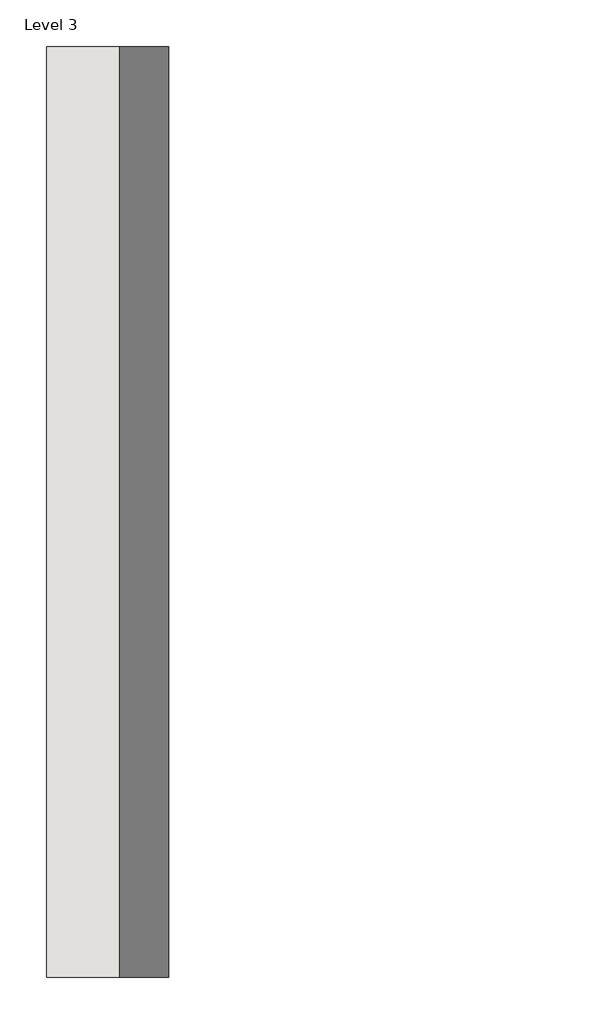
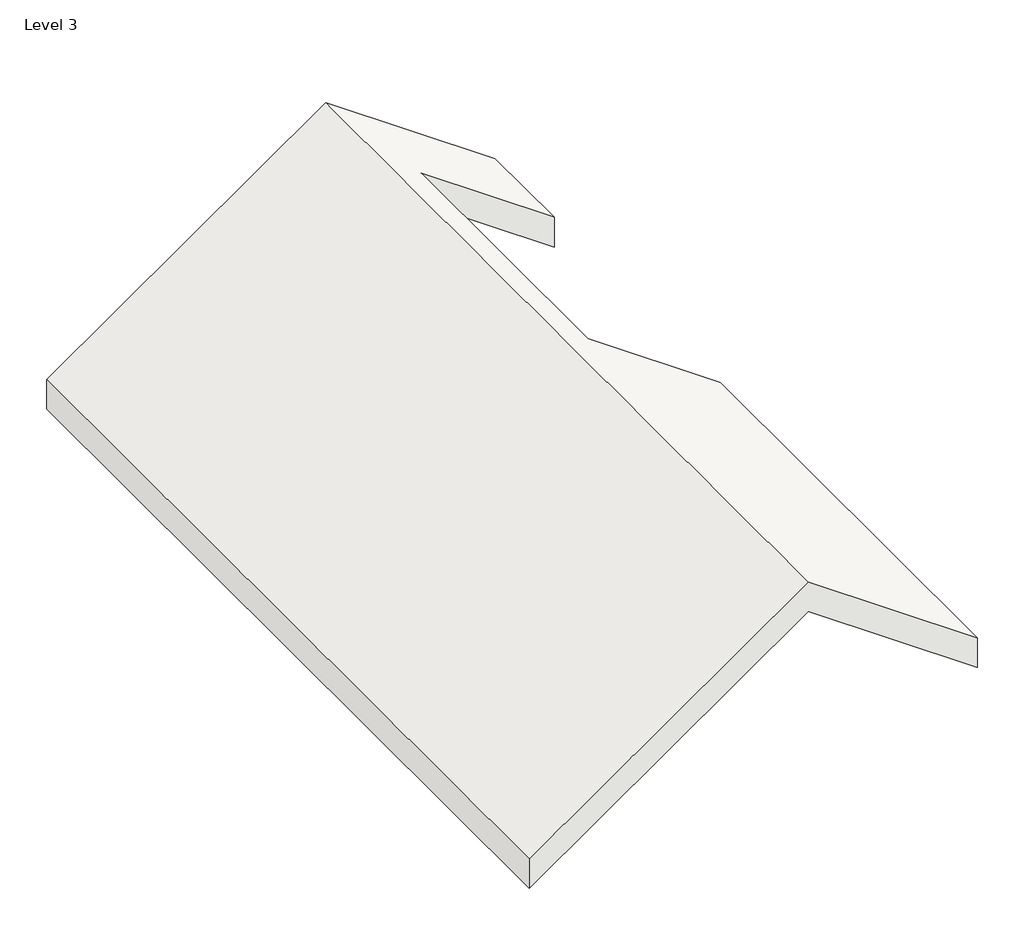
# One storey: 1 roof.
"""IFC4 building model written with IfcOpenShell, lengths in millimetres."""

from ifc_helpers import new_model, si_unit, origin, place, context, project, spatial, faceted_brep, element, save

model = new_model("IFC4")

# Units and contexts
model_context = context("Model", 3, world=origin())
ifc_project = project(units=[si_unit("LENGTHUNIT", "METRE", prefix="MILLI")], contexts=[model_context])

# Site, building, storey
site = spatial("IfcSite", under=ifc_project)
building = spatial("IfcBuilding", under=site)
storey = spatial("IfcBuildingStorey", under=building, Name="Level 3", Elevation=5000.0)

# Roof
placement = place(None, origin())
element("IfcRoof", 1, ObjectType="Generic - 400mm", at=placement, inside=storey, context=model_context, shape_type="Brep", body=[
    faceted_brep([(-6669.0317552, -5566.7477501, 5000.0), (-6669.0317552, 7483.2522499, 5000.0), (-2312.1429511, 7483.2522499, 8050.7263837), (-2312.1429511, -5566.7477501, 8050.7263837), (330.9682448, 7483.2522499, 6200.0), (330.9682448, 5883.2522499, 6200.0), (-1744.0317552, 5883.2522499, 7652.9306418), (-1744.0317552, 1383.2522499, 7652.9306418), (330.9682448, 1383.2522499, 6200.0), (330.9682448, -5566.7477501, 6200.0), (-6669.0317552, 7483.2522499, 5488.3098355), (-6669.0317552, -5566.7477501, 5488.3098355), (-2312.1429511, -5566.7477501, 8539.0362192), (-2312.1429511, 7483.2522499, 8539.0362192), (330.9682448, 7483.2522499, 6688.3098355), (330.9682448, -5566.7477501, 6688.3098355), (330.9682448, 1383.2522499, 6688.3098355), (-1744.0317552, 1383.2522499, 8141.2404773), (-1744.0317552, 5883.2522499, 8141.2404773), (330.9682448, 5883.2522499, 6688.3098355)], [[[0, 1, 2, 3]], [[2, 4, 5, 6, 7, 8, 9, 3]], [[10, 11, 12, 13]], [[14, 13, 12, 15, 16, 17, 18, 19]], [[0, 11, 10, 1]], [[8, 16, 15, 9]], [[4, 14, 19, 5]], [[10, 13, 14, 4, 2, 1]], [[17, 16, 8, 7]], [[18, 17, 7, 6]], [[19, 18, 6, 5]], [[15, 12, 11, 0, 3, 9]]]),
])

save(model, "model.ifc")

# Revit data of these elements
# Type "Generic - 400mm"
#   Layers, outside or top first: 400 mm no material (function 1)
# Element 1 (IfcRoof, "Generic - 400mm")
#   built-in parameter 1001705 = 28.0152 (stored number, unit not read)
#   built-in parameter 1001710 = 33615
#   Phase Created = New Construction
#   Materials on its faces: "Roofing, Tile", "Default Roof"
# Materials
#   "Roofing, Tile": class "Metal", colour RGB 127 127 127, transparency 0, Description = "Clay roofing tile", Cost = 0
#   "Default Roof": colour RGB 0 127 0, transparency 0, Cost = 0
